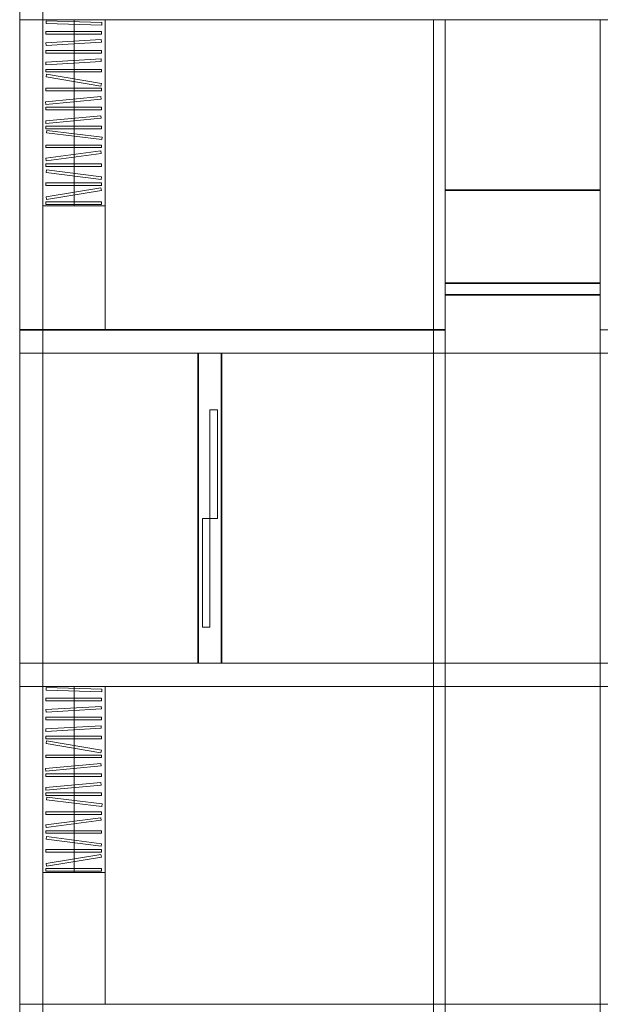
# Model space of a CAD drawing. Units: inches. Extents: x 531915 to 533151, y 849859 to 851471.
# Tile 1 of 7: x 532082 to 532306, y 849859 to 850240. Entities that reach past the tile are written whole.
import ezdxf

# ---------------------------------------------------------------- set-up
doc = ezdxf.new("R2010")
doc.units = ezdxf.units.IN
for name, color, linetype, lineweight in [('A-DOOR', 3, 'Continuous', 18), ('A-FURN', 8, 'Continuous', 13), ('A-NPLT-CNST', 9, 'Continuous', 9), ('A-WALL', 7, 'Continuous', 35)]:
    doc.layers.add(name, color=color, linetype=linetype, lineweight=lineweight)

# ---------------------------------------------------------------- blocks, each defined once
blk = doc.blocks.new('WARDROBE-72')
blk.add_line((12, 0), (12, 72))
for points in [[(24, 0), (24, 72), (0, 72), (0, 0)], [(1.15, 70.47), (1.15, 71.48), (22.64, 71.48), (22.64, 70.47)], [(1.21, 68.56), (1.37, 69.55), (22.58, 66.07), (22.41, 65.07)], [(1.15, 63.15), (1.15, 64.16), (22.64, 64.16), (22.64, 63.15)], [(1.3, 58.13), (1.17, 59.13), (22.48, 61.86), (22.61, 60.86)], [(1.11, 53.59), (1.24, 54.59), (22.54, 51.79), (22.41, 50.79)], [(1.15, 55.83), (1.15, 56.84), (22.64, 56.84), (22.64, 55.83)], [(1.15, 48.51), (1.15, 49.52), (22.64, 49.52), (22.64, 48.51)], [(1.55, 42.84), (1.42, 43.84), (22.76, 46.42), (22.88, 45.42)], [(1.15, 41.19), (1.15, 42.2), (22.64, 42.2), (22.64, 41.19)], [(1.04, 39.13), (1.13, 40.14), (22.52, 38.16), (22.43, 37.15)], [(1.15, 33.87), (1.15, 34.88), (22.64, 34.88), (22.64, 33.87)], [(0.98, 31.76), (1.07, 32.76), (22.47, 30.78), (22.37, 29.78)], [(1.15, 26.55), (1.15, 27.56), (22.64, 27.56), (22.64, 26.55)], [(1.38, 21.1), (1.21, 22.1), (22.4, 25.68), (22.57, 24.68)], [(1.15, 19.23), (1.15, 20.24), (22.64, 20.24), (22.64, 19.23)], [(1.05, 16.46), (1.11, 17.47), (22.56, 16.21), (22.5, 15.2)], [(1.15, 11.91), (1.15, 12.92), (22.64, 12.92), (22.64, 11.91)], [(1.11, 8.97), (1.17, 9.98), (22.62, 8.71), (22.56, 7.7)], [(1.15, 4.59), (1.15, 5.6), (22.64, 5.6), (22.64, 4.59)], [(1.25, 0.42), (1.22, 1.43), (22.7, 2.11), (22.73, 1.1)]]:
    blk.add_lwpolyline(points, close=True)
blk = doc.blocks.new('BALCONY-SLIDER-84')
blk.add_line((2.88, 84), (2.88, 0))
for points in [[(2.88, 84), (5.76, 84), (5.76, 41.94), (2.88, 41.94)], [(2.88, 41.94), (0, 41.94), (0, 0), (2.88, 0)]]:
    blk.add_lwpolyline(points, close=True)

msp = doc.modelspace()

# ---------------------------------------------------------------- linework, layer by layer
at = {"layer": 'A-FURN'}
for p, q in [((532114.8048, 850168.374), (532114.8048, 850120.374)), ((532114.8048, 849910.374), (532114.8048, 849859.374))]:
    msp.add_line(p, q, dxfattribs=at)
at = {"layer": 'A-NPLT-CNST'}
for p, direction in [((532081.8048, 850249.374), (0, -1)), ((532081.8048, 850249.374), (1, 0)), ((532090.8048, 850249.374), (0, -1)), ((532442.8048, 850249.374), (0, -1)), ((532451.8048, 850249.374), (0, -1)), ((532081.8048, 850240.374), (1, 0)), ((532241.8048, 850240.374), (0, -1)), ((532246.3048, 850240.374), (0, -1)), ((532306.3048, 850240.374), (0, -1)), ((532310.8048, 850240.374), (0, -1)), ((532306.3048, 850120.374), (1, 0)), ((532081.8048, 850111.374), (1, 0)), ((532081.8048, 849991.374), (1, 0)), ((532081.8048, 849982.374), (1, 0)), ((532081.8048, 849859.374), (1, 0))]:
    msp.add_ray(p, direction, dxfattribs=at)
at = {"layer": 'A-WALL'}
for p, q in [((532246.3048, 850174.374), (532306.3048, 850174.374)), ((532246.3048, 850138.374), (532306.3048, 850138.374)), ((532246.3048, 850133.874), (532306.3048, 850133.874)), ((532081.8048, 850120.374), (532246.3048, 850120.374)), ((532150.8048, 850111.374), (532150.8048, 849991.374)), ((532159.8048, 850111.374), (532159.8048, 849991.374))]:
    msp.add_line(p, q, dxfattribs=at)

# ---------------------------------------------------------------- block references
at = {"layer": 'A-DOOR'}
msp.add_blockref('BALCONY-SLIDER-84', (532152.4675, 850005.374), dxfattribs=at)
at = {"layer": 'A-FURN', "extrusion": (0, 0, -1), "zscale": -1, "rotation": 180}
for p in [(-532090.8048, 850240.374), (-532090.8048, 849982.374)]:
    msp.add_blockref('WARDROBE-72', p, dxfattribs=at)

doc.saveas('drawing.dxf')
